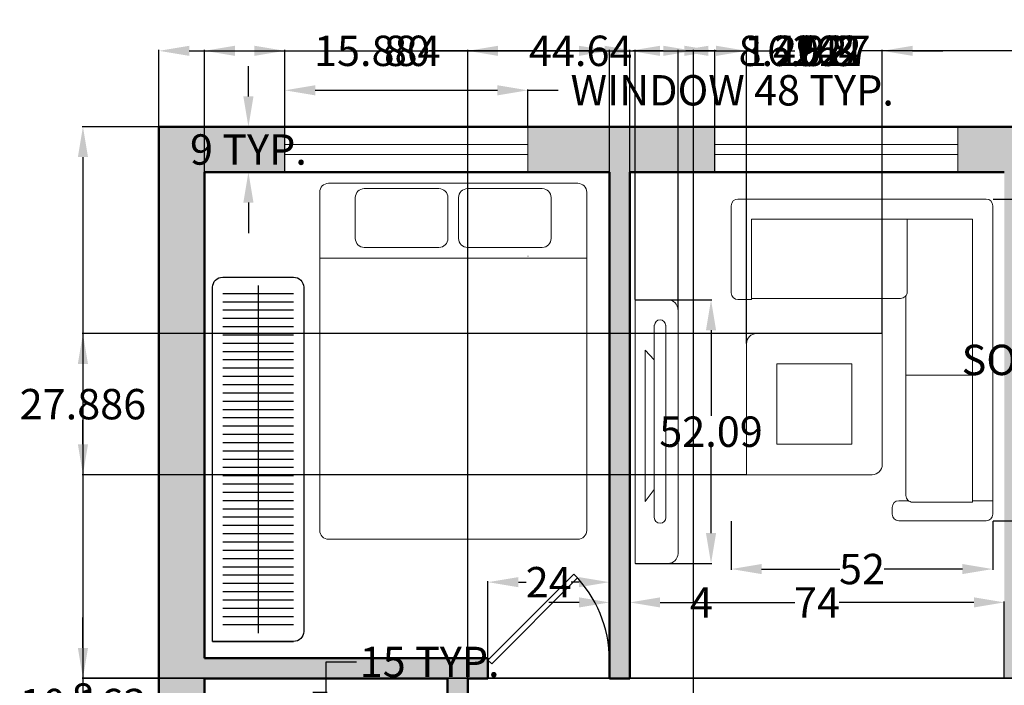
# Model space of a CAD drawing. Units: inches. Extents: x -11 to 341, y -300 to 41.
# Tile 3 of 5: x -3 to 192, y -91 to 41. Entities that reach past the tile are written whole.
import ezdxf

# ---------------------------------------------------------------- set-up
doc = ezdxf.new("R2010")
doc.units = ezdxf.units.IN
doc.header["$MEASUREMENT"] = 0
for name, color, linetype, lineweight in [('A-ANNO-DIMS', 2, 'Continuous', 18), ('A-DOOR', 3, 'Continuous', 25), ('A-FLOR-CASE', 8, 'Continuous', 25), ('A-FURN', 8, 'Continuous', 18), ('A-GLAZ', 4, 'Continuous', 18), ('A-WALL', 7, 'Continuous', 50), ('A-WALL-PATT', 251, 'Continuous', 13)]:
    doc.layers.add(name, color=color, linetype=linetype, lineweight=lineweight)
doc.styles.get("Standard").update_dxf_attribs({"font": 'arial.ttf'})
doc.dimstyles.get("Standard").update_dxf_attribs({"dimtxt": 6, "dimasz": 6, "dimexe": 0.18, "dimexo": 0.0625, "dimgap": 0.09, "dimtad": 0, "dimtih": 1, "dimtoh": 1, "dimdec": 0, "dimzin": 0, "dimdsep": 46, "dimlunit": 4, "dimtxsty": 'Standard', "dimcen": 0.09, "dimadec": 0, "dimazin": 0, "dimtfac": 1, "dimtdec": 0, "dimtofl": 0, "dimtmove": 0, "dimatfit": 3, "dimfxl": 1, "dimtolj": 1, "dimtzin": 0, "dimarcsym": 0})

# ---------------------------------------------------------------- blocks, each defined once
blk = doc.blocks.new('*U14')
for p, q in [((0, 0), (0, -6)), ((40, 0), (40, -6))]:
    blk.add_line(p, q)
blk.add_lwpolyline([(0, 0), (28.28, 28.28), (29.52, 27.05), (1.24, -1.24)], close=True)
blk.add_arc((0, 0), 40, 0, 45)
blk = doc.blocks.new('Bed - Queen')
for p, q in [((2, 0), (57.99999, 0)), ((0, -78.00003), (0, -2)), ((9.99999, -1.2), (26.79998, -1.2)), ((33.19999, -1.2), (49.99999, -1.2)), ((59.99999, -2), (59.99999, -78.00003)), ((7.99999, -12.4), (7.99999, -3.2)), ((28.79998, -3.2), (28.79998, -12.4)), ((31.19999, -12.4), (31.19999, -3.2)), ((51.99999, -3.2), (51.99999, -12.4)), ((9.99999, -14.4), (26.79998, -14.4)), ((33.19999, -14.4), (49.99999, -14.4)), ((59.99999, -16.8), (0, -16.8)), ((46.8, -16.4), (46.79936, -16.4)), ((57.99999, -80.00003), (2, -80.00003))]:
    blk.add_line(p, q)
for centre, start, end in [((2, -2), 90, 180), ((57.99999, -2), 0, 90), ((9.99999, -3.2), 90, 180), ((26.79998, -3.2), 0, 90), ((33.19999, -3.2), 90, 180), ((49.99999, -3.2), 0, 90), ((9.99999, -12.4), 180, 270), ((26.79998, -12.4), 270, 0), ((33.19999, -12.4), 180, 270), ((49.99999, -12.4), 270, 0), ((2, -78.00003), 180, 270), ((57.99999, -78.00003), 270, 0)]:
    blk.add_arc(centre, 2, start, end)
blk = doc.blocks.new('L Sofa')
for p, q in [((2, 30), (72, 30)), ((72, 30), (76, 30)), ((0, 24), (0, 28)), ((78, 28), (78, -54)), ((0, 2), (0, 24)), ((72, 24), (6, 24)), ((6, 24), (6, 0)), ((72, 24), (52.59, 24)), ((72, -60), (72, 24)), ((72, -22.55), (72, 24)), ((6, 0), (2, 0)), ((52.09, -22.55), (52.09, 1.16)), ((52.59, -22.55), (72, -22.55)), ((78, -54), (78, -60)), ((50, -60), (52.83, -60)), ((78, -60), (72, -60)), ((78, -60), (78, -64)), ((48, -64), (48, -62)), ((54, -66), (50, -66)), ((76, -66), (54, -66))]:
    blk.add_line(p, q)
for points in [[(6, 24), (52.48, 24), (52.48, 2.35, -0.414214), (50.48, 0.35), (6, 0.35)], [(72, -22.55), (52.09, -22.55), (52.09, -58.44, 0.414214), (54.09, -60.44), (72, -60.44)]]:
    blk.add_lwpolyline(points, format="xyb", close=True)
for centre, start, end in [((2, 28), 90, 180), ((76, 28), 0, 90), ((2, 2), 180, 270), ((50, -62), 90, 180), ((50, -64), 180, 270), ((76, -64), 270, 0)]:
    blk.add_arc(centre, 2, start, end)
blk = doc.blocks.new('WIN-48IN')
for p, q in [((0, 0), (0, 9)), ((48, 9), (48, 0)), ((0, 5.5), (48, 5.5)), ((0, 3.5), (48, 3.5))]:
    blk.add_line(p, q)
blk = doc.blocks.new('WARDROBE-HANGING-RAIL')
for p, q in [((7, 68.73), (7, 0)), ((14, 67.09), (0, 67.09)), ((14, 65.45), (0, 65.45)), ((14, 63.82), (0, 63.82)), ((14, 62.18), (0, 62.18)), ((14, 60.55), (0, 60.55)), ((14, 58.91), (0, 58.91)), ((14, 57.27), (0, 57.27)), ((14, 55.64), (0, 55.64)), ((14, 54), (0, 54)), ((14, 52.36), (0, 52.36)), ((14, 50.73), (0, 50.73)), ((14, 49.09), (0, 49.09)), ((14, 47.45), (0, 47.45)), ((14, 45.82), (0, 45.82)), ((14, 44.18), (0, 44.18)), ((14, 42.55), (0, 42.55)), ((14, 40.91), (0, 40.91)), ((14, 39.27), (0, 39.27)), ((14, 37.64), (0, 37.64)), ((14, 36), (0, 36)), ((14, 34.36), (0, 34.36)), ((14, 32.73), (0, 32.73)), ((14, 31.09), (0, 31.09)), ((14, 29.45), (0, 29.45)), ((14, 27.82), (0, 27.82)), ((14, 26.18), (0, 26.18)), ((14, 24.55), (0, 24.55)), ((14, 22.91), (0, 22.91)), ((14, 21.27), (0, 21.27)), ((14, 19.64), (0, 19.64)), ((14, 18), (0, 18)), ((14, 16.36), (0, 16.36)), ((14, 14.73), (0, 14.73)), ((14, 13.09), (0, 13.09)), ((14, 11.45), (0, 11.45)), ((14, 9.82), (0, 9.82)), ((14, 8.18), (0, 8.18)), ((14, 6.55), (0, 6.55)), ((14, 4.91), (0, 4.91)), ((14, 3.27), (0, 3.27)), ((14, 1.64), (0, 1.64))]:
    blk.add_line(p, q)
blk = doc.blocks.new('*D19')
at = {"layer": 'A-ANNO-DIMS', "color": 0, "lineweight": -2, "transparency": 16777216}
for p, q in [((49.45, 19.46), (49.45, 26.78)), ((55.45, 26.6), (91.45, 26.6)), ((97.45, 19.46), (97.45, 26.78)), ((97.45, 26.6), (103.45, 26.6))]:
    blk.add_line(p, q, dxfattribs=at)
at = {"layer": 'A-ANNO-DIMS', "color": 0, "transparency": 16777216}
for points in [[(55.45, 27.6), (55.45, 25.6), (49.45, 26.6)], [(91.45, 27.6), (91.45, 25.6), (97.45, 26.6)]]:
    blk.add_solid(points, dxfattribs=at)
at = {"layer": 'Defpoints', "color": 0, "transparency": 16777216}
for p in [(97.45, 26.6), (49.45, 19.4), (97.45, 19.4)]:
    blk.add_point(p, dxfattribs=at)
at = {"layer": 'A-ANNO-DIMS', "color": 0, "transparency": 16777216, "insert": (137.82, 26.6), "char_height": 6, "attachment_point": 5}
blk.add_mtext('\\A1;WINDOW 48 TYP.', dxfattribs=at)
blk = doc.blocks.new('*D20')
at = {"layer": 'A-ANNO-DIMS', "color": 0, "lineweight": -2, "transparency": 16777216}
for p, q in [((42.25, 25.4), (42.25, 31.4)), ((49.39, 19.4), (42.07, 19.4)), ((49.39, 10.4), (42.07, 10.4)), ((42.25, 4.4), (42.25, -1.6))]:
    blk.add_line(p, q, dxfattribs=at)
at = {"layer": 'A-ANNO-DIMS', "color": 0, "transparency": 16777216}
for points in [[(41.25, 25.4), (43.25, 25.4), (42.25, 19.4)], [(41.25, 4.4), (43.25, 4.4), (42.25, 10.4)]]:
    blk.add_solid(points, dxfattribs=at)
at = {"layer": 'Defpoints', "color": 0, "transparency": 16777216}
for p in [(42.25, 19.4), (49.45, 19.4), (49.45, 10.4)]:
    blk.add_point(p, dxfattribs=at)
at = {"layer": 'A-ANNO-DIMS', "color": 0, "transparency": 16777216, "insert": (42.25, 14.9), "char_height": 6, "attachment_point": 5}
blk.add_mtext('\\A1;9 TYP.', dxfattribs=at)
blk = doc.blocks.new('*D32')
at = {"layer": 'A-ANNO-DIMS', "color": 0, "lineweight": -2, "transparency": 16777216}
for p, q in [((57.63, -92.36), (57.63, -86.36)), ((57.63, -86.36), (63.63, -86.36)), ((54.99, -92.36), (57.81, -92.36)), ((57.63, -101.17), (57.63, -98.36)), ((54.99, -107.17), (57.81, -107.17))]:
    blk.add_line(p, q, dxfattribs=at)
at = {"layer": 'A-ANNO-DIMS', "color": 0, "transparency": 16777216}
for points in [[(56.63, -98.36), (58.63, -98.36), (57.63, -92.36)], [(56.63, -101.17), (58.63, -101.17), (57.63, -107.17)]]:
    blk.add_solid(points, dxfattribs=at)
at = {"layer": 'Defpoints', "color": 0, "transparency": 16777216}
for p in [(54.93, -92.36), (57.63, -92.36), (54.93, -107.17)]:
    blk.add_point(p, dxfattribs=at)
at = {"layer": 'A-ANNO-DIMS', "color": 0, "transparency": 16777216, "insert": (78.05, -86.36), "char_height": 6, "attachment_point": 5}
blk.add_mtext('\\A1;15 TYP.', dxfattribs=at)
blk = doc.blocks.new('*D41')
at = {"layer": 'A-ANNO-DIMS', "color": 0, "lineweight": -2, "transparency": 16777216}
for p, q in [((189.35, 5.11), (199, 5.11)), ((198.82, -0.89), (198.82, -23.48)), ((198.82, -52.47), (198.82, -29.87)), ((189.35, -58.47), (199, -58.47))]:
    blk.add_line(p, q, dxfattribs=at)
at = {"layer": 'A-ANNO-DIMS', "color": 0, "transparency": 16777216}
for points in [[(197.82, -0.89), (199.82, -0.89), (198.82, 5.11)], [(197.82, -52.47), (199.82, -52.47), (198.82, -58.47)]]:
    blk.add_solid(points, dxfattribs=at)
at = {"layer": 'Defpoints', "color": 0, "transparency": 16777216}
for p in [(189.29, 5.11), (198.82, 5.11), (189.29, -58.47)]:
    blk.add_point(p, dxfattribs=at)
at = {"layer": 'A-ANNO-DIMS', "color": 0, "transparency": 16777216, "insert": (198.82, -26.68), "char_height": 6, "attachment_point": 5}
blk.add_mtext('\\A1;SOFA 64', dxfattribs=at)
blk = doc.blocks.new('*D42')
at = {"layer": 'A-ANNO-DIMS', "color": 0, "lineweight": -2, "transparency": 16777216}
for p, q in [((137.63, -58.53), (137.63, -68.19)), ((189.29, -58.53), (189.29, -68.19)), ((143.63, -68.01), (159.1, -68.01)), ((183.29, -68.01), (167.81, -68.01))]:
    blk.add_line(p, q, dxfattribs=at)
at = {"layer": 'A-ANNO-DIMS', "color": 0, "transparency": 16777216}
for points in [[(143.63, -67.01), (143.63, -69.01), (137.63, -68.01)], [(183.29, -67.01), (183.29, -69.01), (189.29, -68.01)]]:
    blk.add_solid(points, dxfattribs=at)
at = {"layer": 'Defpoints', "color": 0, "transparency": 16777216}
for p in [(137.63, -58.47), (189.29, -58.47), (189.29, -68.01)]:
    blk.add_point(p, dxfattribs=at)
at = {"layer": 'A-ANNO-DIMS', "color": 0, "transparency": 16777216, "insert": (163.46, -68.01), "char_height": 6, "attachment_point": 5}
blk.add_mtext('\\A1;52', dxfattribs=at)
blk = doc.blocks.new('*D45')
at = {"layer": 'A-ANNO-DIMS', "color": 0, "lineweight": -2, "transparency": 16777216}
for p, q in [((24.57, 19.46), (24.57, 34.58)), ((30.57, 34.4), (149.81, 34.4)), ((282.57, 34.4), (163.32, 34.4)), ((288.57, 19.46), (288.57, 34.58))]:
    blk.add_line(p, q, dxfattribs=at)
at = {"layer": 'A-ANNO-DIMS', "color": 0, "transparency": 16777216}
for points in [[(30.57, 35.4), (30.57, 33.4), (24.57, 34.4)], [(282.57, 35.4), (282.57, 33.4), (288.57, 34.4)]]:
    blk.add_solid(points, dxfattribs=at)
at = {"layer": 'Defpoints', "color": 0, "transparency": 16777216}
for p in [(288.57, 34.4), (24.57, 19.4), (288.57, 19.4)]:
    blk.add_point(p, dxfattribs=at)
at = {"layer": 'A-ANNO-DIMS', "color": 0, "transparency": 16777216, "insert": (156.57, 34.4), "char_height": 6, "attachment_point": 5}
blk.add_mtext('\\A1;264', dxfattribs=at)
blk = doc.blocks.new('*D46')
at = {"layer": 'A-ANNO-DIMS', "color": 0, "lineweight": -2, "transparency": 16777216}
for p, q in [((24.5, 19.4), (9.38, 19.4)), ((9.56, 13.4), (9.56, -127.45)), ((9.56, -274.6), (9.56, -133.76)), ((24.5, -280.6), (9.38, -280.6))]:
    blk.add_line(p, q, dxfattribs=at)
at = {"layer": 'A-ANNO-DIMS', "color": 0, "transparency": 16777216}
for points in [[(8.56, 13.4), (10.56, 13.4), (9.56, 19.4)], [(8.56, -274.6), (10.56, -274.6), (9.56, -280.6)]]:
    blk.add_solid(points, dxfattribs=at)
at = {"layer": 'Defpoints', "color": 0, "transparency": 16777216}
for p in [(9.56, 19.4), (24.57, 19.4), (24.57, -280.6)]:
    blk.add_point(p, dxfattribs=at)
at = {"layer": 'A-ANNO-DIMS', "color": 0, "transparency": 16777216, "insert": (9.56, -130.6), "char_height": 6, "attachment_point": 5}
blk.add_mtext('\\A1;300', dxfattribs=at)
blk = doc.blocks.new('*D47')
at = {"layer": 'A-ANNO-DIMS', "color": 0, "lineweight": -2, "transparency": 16777216}
for p, q in [((33.57, 10.46), (33.57, 34.58)), ((39.57, 34.4), (43.45, 34.4)), ((49.45, 10.46), (49.45, 34.58)), ((49.45, 34.4), (55.45, 34.4))]:
    blk.add_line(p, q, dxfattribs=at)
at = {"layer": 'A-ANNO-DIMS', "color": 0, "transparency": 16777216}
for points in [[(39.57, 35.4), (39.57, 33.4), (33.57, 34.4)], [(43.45, 35.4), (43.45, 33.4), (49.45, 34.4)]]:
    blk.add_solid(points, dxfattribs=at)
at = {"layer": 'Defpoints', "color": 0, "transparency": 16777216}
for p in [(49.45, 34.4), (33.57, 10.4), (49.45, 10.4)]:
    blk.add_point(p, dxfattribs=at)
at = {"layer": 'A-ANNO-DIMS', "color": 0, "transparency": 16777216, "insert": (67.7, 34.4), "char_height": 6, "attachment_point": 5}
blk.add_mtext('\\A1;15.884', dxfattribs=at)
blk = doc.blocks.new('*D48')
at = {"layer": 'A-ANNO-DIMS', "color": 0, "lineweight": -2, "transparency": 16777216}
for p, q in [((117.57, 10.46), (117.57, 34.58)), ((123.57, 34.4), (128.39, 34.4)), ((134.39, 10.46), (134.39, 34.58)), ((134.39, 34.4), (140.39, 34.4))]:
    blk.add_line(p, q, dxfattribs=at)
at = {"layer": 'A-ANNO-DIMS', "color": 0, "transparency": 16777216}
for points in [[(123.57, 35.4), (123.57, 33.4), (117.57, 34.4)], [(128.39, 35.4), (128.39, 33.4), (134.39, 34.4)]]:
    blk.add_solid(points, dxfattribs=at)
at = {"layer": 'Defpoints', "color": 0, "transparency": 16777216}
for p in [(134.39, 34.4), (117.57, 10.4), (134.39, 10.4)]:
    blk.add_point(p, dxfattribs=at)
at = {"layer": 'A-ANNO-DIMS', "color": 0, "transparency": 16777216, "insert": (152.65, 34.4), "char_height": 6, "attachment_point": 5}
blk.add_mtext('\\A1;16.827', dxfattribs=at)
blk = doc.blocks.new('*D54')
at = {"layer": 'A-ANNO-DIMS', "color": 0, "lineweight": -2, "transparency": 16777216}
for p, q in [((33.57, -85.54), (33.57, 34.58)), ((39.57, 34.4), (69.18, 34.4)), ((107.57, 34.4), (77.95, 34.4)), ((113.57, -85.54), (113.57, 34.58))]:
    blk.add_line(p, q, dxfattribs=at)
at = {"layer": 'A-ANNO-DIMS', "color": 0, "transparency": 16777216}
for points in [[(39.57, 35.4), (39.57, 33.4), (33.57, 34.4)], [(107.57, 35.4), (107.57, 33.4), (113.57, 34.4)]]:
    blk.add_solid(points, dxfattribs=at)
at = {"layer": 'Defpoints', "color": 0, "transparency": 16777216}
for p in [(113.57, 34.4), (33.57, -85.6), (113.57, -85.6)]:
    blk.add_point(p, dxfattribs=at)
at = {"layer": 'A-ANNO-DIMS', "color": 0, "transparency": 16777216, "insert": (73.57, 34.4), "char_height": 6, "attachment_point": 5}
blk.add_mtext('\\A1;80', dxfattribs=at)
blk = doc.blocks.new('*D55')
at = {"layer": 'A-ANNO-DIMS', "color": 0, "lineweight": -2, "transparency": 16777216}
for p, q in [((107.57, -74.6), (101.57, -74.6)), ((113.57, -89.54), (113.57, -74.42)), ((117.57, -89.54), (117.57, -74.42)), ((123.57, -74.6), (129.57, -74.6))]:
    blk.add_line(p, q, dxfattribs=at)
at = {"layer": 'A-ANNO-DIMS', "color": 0, "transparency": 16777216}
for points in [[(107.57, -73.6), (107.57, -75.6), (113.57, -74.6)], [(123.57, -73.6), (123.57, -75.6), (117.57, -74.6)]]:
    blk.add_solid(points, dxfattribs=at)
at = {"layer": 'Defpoints', "color": 0, "transparency": 16777216}
for p in [(117.57, -74.6), (113.57, -89.6), (117.57, -89.6)]:
    blk.add_point(p, dxfattribs=at)
at = {"layer": 'A-ANNO-DIMS', "color": 0, "transparency": 16777216, "insert": (131.73, -74.6), "char_height": 6, "attachment_point": 5}
blk.add_mtext('\\A1;4', dxfattribs=at)
blk = doc.blocks.new('*D56')
at = {"layer": 'A-ANNO-DIMS', "color": 0, "lineweight": -2, "transparency": 16777216}
for p, q in [((117.57, -89.54), (117.57, -74.42)), ((123.57, -74.6), (150.21, -74.6)), ((185.57, -74.6), (158.92, -74.6)), ((191.57, -89.54), (191.57, -74.42))]:
    blk.add_line(p, q, dxfattribs=at)
at = {"layer": 'A-ANNO-DIMS', "color": 0, "transparency": 16777216}
for points in [[(123.57, -73.6), (123.57, -75.6), (117.57, -74.6)], [(185.57, -73.6), (185.57, -75.6), (191.57, -74.6)]]:
    blk.add_solid(points, dxfattribs=at)
at = {"layer": 'Defpoints', "color": 0, "transparency": 16777216}
for p in [(191.57, -74.6), (117.57, -89.6), (191.57, -89.6)]:
    blk.add_point(p, dxfattribs=at)
at = {"layer": 'A-ANNO-DIMS', "color": 0, "transparency": 16777216, "insert": (154.57, -74.6), "char_height": 6, "attachment_point": 5}
blk.add_mtext('\\A1;74', dxfattribs=at)
blk = doc.blocks.new('*D62')
at = {"layer": 'A-ANNO-DIMS', "color": 0, "lineweight": -2, "transparency": 16777216}
for p, q in [((85.57, -175.54), (85.57, 34.58)), ((91.57, 34.4), (150.16, 34.4)), ((221.57, 34.4), (162.97, 34.4)), ((227.57, -175.54), (227.57, 34.58))]:
    blk.add_line(p, q, dxfattribs=at)
at = {"layer": 'A-ANNO-DIMS', "color": 0, "transparency": 16777216}
for points in [[(91.57, 35.4), (91.57, 33.4), (85.57, 34.4)], [(221.57, 35.4), (221.57, 33.4), (227.57, 34.4)]]:
    blk.add_solid(points, dxfattribs=at)
at = {"layer": 'Defpoints', "color": 0, "transparency": 16777216}
for p in [(227.57, 34.4), (85.57, -175.6), (227.57, -175.6)]:
    blk.add_point(p, dxfattribs=at)
at = {"layer": 'A-ANNO-DIMS', "color": 0, "transparency": 16777216, "insert": (156.57, 34.4), "char_height": 6, "attachment_point": 5}
blk.add_mtext('\\A1;142', dxfattribs=at)
blk = doc.blocks.new('*D66')
at = {"layer": 'A-ANNO-DIMS', "color": 0, "lineweight": -2, "transparency": 16777216}
for p, q in [((9.563121, -83.603265), (9.563121, -77.603265)), ((231.502621, -89.603265), (9.383121, -89.603265)), ((231.502621, -97.603265), (9.383121, -97.603265)), ((9.563121, -103.603265), (9.563121, -109.603265))]:
    blk.add_line(p, q, dxfattribs=at)
at = {"layer": 'A-ANNO-DIMS', "color": 0, "transparency": 16777216}
for points in [[(8.563121, -83.603265), (10.563121, -83.603265), (9.563121, -89.603265)], [(8.563121, -103.603265), (10.563121, -103.603265), (9.563121, -97.603265)]]:
    blk.add_solid(points, dxfattribs=at)
at = {"layer": 'Defpoints', "color": 0, "transparency": 16777216}
for p in [(231.565121, -89.603265), (9.563121, -97.603265), (231.565121, -97.603265)]:
    blk.add_point(p, dxfattribs=at)
at = {"layer": 'A-ANNO-DIMS', "color": 0, "transparency": 16777216, "insert": (9.563121, -93.603265), "char_height": 6, "attachment_point": 5}
blk.add_mtext('\\A1;8', dxfattribs=at)
blk = doc.blocks.new('*D68')
at = {"layer": 'A-ANNO-DIMS', "color": 0, "lineweight": -2, "transparency": 16777216}
for p, q in [((89.57, -85.54), (89.57, -70.42)), ((95.57, -70.6), (97.14, -70.6)), ((107.57, -70.6), (105.99, -70.6)), ((113.57, -85.54), (113.57, -70.42))]:
    blk.add_line(p, q, dxfattribs=at)
at = {"layer": 'A-ANNO-DIMS', "color": 0, "transparency": 16777216}
for points in [[(95.57, -69.6), (95.57, -71.6), (89.57, -70.6)], [(107.57, -69.6), (107.57, -71.6), (113.57, -70.6)]]:
    blk.add_solid(points, dxfattribs=at)
at = {"layer": 'Defpoints', "color": 0, "transparency": 16777216}
for p in [(113.57, -70.6), (89.57, -85.6), (113.57, -85.6)]:
    blk.add_point(p, dxfattribs=at)
at = {"layer": 'A-ANNO-DIMS', "color": 0, "transparency": 16777216, "insert": (101.57, -70.6), "char_height": 6, "attachment_point": 5}
blk.add_mtext('\\A1;24', dxfattribs=at)
blk = doc.blocks.new('*D78')
at = {"layer": 'A-ANNO-DIMS', "color": 0, "lineweight": -2, "transparency": 16777216}
for p, q in [((118.69, -14.81), (133.81, -14.81)), ((133.63, -20.81), (133.63, -37.71)), ((133.63, -60.9), (133.63, -44.01)), ((118.69, -66.9), (133.81, -66.9))]:
    blk.add_line(p, q, dxfattribs=at)
at = {"layer": 'A-ANNO-DIMS', "color": 0, "transparency": 16777216}
for points in [[(132.63, -20.81), (134.63, -20.81), (133.63, -14.81)], [(132.63, -60.9), (134.63, -60.9), (133.63, -66.9)]]:
    blk.add_solid(points, dxfattribs=at)
at = {"layer": 'Defpoints', "color": 0, "transparency": 16777216}
for p in [(118.63, -14.81), (118.63, -66.9), (133.63, -66.9)]:
    blk.add_point(p, dxfattribs=at)
at = {"layer": 'A-ANNO-DIMS', "color": 0, "transparency": 16777216, "insert": (133.63, -40.86), "char_height": 6, "attachment_point": 5}
blk.add_mtext('\\A1;52.09', dxfattribs=at)
blk = doc.blocks.new('*D79')
at = {"layer": 'A-ANNO-DIMS', "color": 0, "lineweight": -2, "transparency": 16777216}
for p, q in [((112.63, 34.4), (106.63, 34.4)), ((118.63, -14.75), (118.63, 34.58)), ((127.12, -16.75), (127.12, 34.58)), ((133.12, 34.4), (139.12, 34.4))]:
    blk.add_line(p, q, dxfattribs=at)
at = {"layer": 'A-ANNO-DIMS', "color": 0, "transparency": 16777216}
for points in [[(112.63, 35.4), (112.63, 33.4), (118.63, 34.4)], [(133.12, 35.4), (133.12, 33.4), (127.12, 34.4)]]:
    blk.add_solid(points, dxfattribs=at)
at = {"layer": 'Defpoints', "color": 0, "transparency": 16777216}
for p in [(127.12, 34.4), (118.63, -14.81), (127.12, -16.81)]:
    blk.add_point(p, dxfattribs=at)
at = {"layer": 'A-ANNO-DIMS', "color": 0, "transparency": 16777216, "insert": (149.3, 34.4), "char_height": 6, "attachment_point": 5}
blk.add_mtext('\\A1;8.492', dxfattribs=at)
blk = doc.blocks.new('*D80')
at = {"layer": 'A-ANNO-DIMS', "color": 0, "lineweight": -2, "transparency": 16777216}
for p, q in [((134.645775, 34.398735), (128.645775, 34.398735)), ((140.645775, -23.409984), (140.645775, 34.578735)), ((167.445879, -21.409984), (167.445879, 34.578735)), ((173.445879, 34.398735), (179.445879, 34.398735))]:
    blk.add_line(p, q, dxfattribs=at)
at = {"layer": 'A-ANNO-DIMS', "color": 0, "transparency": 16777216}
for points in [[(134.645775, 35.398735), (134.645775, 33.398735), (140.645775, 34.398735)], [(173.445879, 35.398735), (173.445879, 33.398735), (167.445879, 34.398735)]]:
    blk.add_solid(points, dxfattribs=at)
at = {"layer": 'Defpoints', "color": 0, "transparency": 16777216}
for p in [(167.445879, 34.398735), (167.445879, -21.472484), (140.645775, -23.472484)]:
    blk.add_point(p, dxfattribs=at)
at = {"layer": 'A-ANNO-DIMS', "color": 0, "transparency": 16777216, "insert": (154.045827, 34.398735), "char_height": 6, "attachment_point": 5}
blk.add_mtext('\\A1;26.8', dxfattribs=at)
blk = doc.blocks.new('*D81')
at = {"layer": 'A-ANNO-DIMS', "color": 0, "lineweight": -2, "transparency": 16777216}
for p, q in [((167.38, -21.47), (9.38, -21.47)), ((9.56, -27.47), (9.56, -32.26)), ((9.56, -43.36), (9.56, -38.57)), ((140.58, -49.36), (9.38, -49.36))]:
    blk.add_line(p, q, dxfattribs=at)
at = {"layer": 'A-ANNO-DIMS', "color": 0, "transparency": 16777216}
for points in [[(8.56, -27.47), (10.56, -27.47), (9.56, -21.47)], [(8.56, -43.36), (10.56, -43.36), (9.56, -49.36)]]:
    blk.add_solid(points, dxfattribs=at)
at = {"layer": 'Defpoints', "color": 0, "transparency": 16777216}
for p in [(9.56, -21.47), (167.45, -21.47), (140.65, -49.36)]:
    blk.add_point(p, dxfattribs=at)
at = {"layer": 'A-ANNO-DIMS', "color": 0, "transparency": 16777216, "insert": (9.56, -35.42), "char_height": 6, "attachment_point": 5}
blk.add_mtext('\\A1;27.886', dxfattribs=at)
blk = doc.blocks.new('*D84')
at = {"layer": 'A-ANNO-DIMS', "color": 0, "lineweight": -2, "transparency": 16777216}
for p, q in [((9.56, -83.6), (9.56, -77.6)), ((279.5, -89.6), (9.38, -89.6)), ((267.79, -99.77), (9.38, -99.77)), ((9.56, -105.77), (9.56, -111.77))]:
    blk.add_line(p, q, dxfattribs=at)
at = {"layer": 'A-ANNO-DIMS', "color": 0, "transparency": 16777216}
for points in [[(8.56, -83.6), (10.56, -83.6), (9.56, -89.6)], [(8.56, -105.77), (10.56, -105.77), (9.56, -99.77)]]:
    blk.add_solid(points, dxfattribs=at)
at = {"layer": 'Defpoints', "color": 0, "transparency": 16777216}
for p in [(9.56, -89.6), (279.57, -89.6), (267.86, -99.77)]:
    blk.add_point(p, dxfattribs=at)
at = {"layer": 'A-ANNO-DIMS', "color": 0, "transparency": 16777216, "insert": (9.56, -94.68), "char_height": 6, "attachment_point": 5}
blk.add_mtext('\\A1;10.163', dxfattribs=at)
blk = doc.blocks.new('*D85')
at = {"layer": 'A-ANNO-DIMS', "color": 0, "lineweight": -2, "transparency": 16777216}
for p, q in [((85.57, -127.54), (85.57, 34.58)), ((91.57, 34.4), (97.56, 34.4)), ((124.2, 34.4), (118.21, 34.4)), ((130.2, -129.38), (130.2, 34.58))]:
    blk.add_line(p, q, dxfattribs=at)
at = {"layer": 'A-ANNO-DIMS', "color": 0, "transparency": 16777216}
for points in [[(91.57, 35.4), (91.57, 33.4), (85.57, 34.4)], [(124.2, 35.4), (124.2, 33.4), (130.2, 34.4)]]:
    blk.add_solid(points, dxfattribs=at)
at = {"layer": 'Defpoints', "color": 0, "transparency": 16777216}
for p in [(130.2, 34.4), (85.57, -127.6), (130.2, -129.44)]:
    blk.add_point(p, dxfattribs=at)
at = {"layer": 'A-ANNO-DIMS', "color": 0, "transparency": 16777216, "insert": (107.88, 34.4), "char_height": 6, "attachment_point": 5}
blk.add_mtext('\\A1;44.64', dxfattribs=at)

msp = doc.modelspace()

# ---------------------------------------------------------------- hatches: boundary and pattern name
at = {"layer": 'A-WALL-PATT'}
h = msp.add_hatch(color=256, dxfattribs=at)
h.dxf.hatch_style = 1
h.paths.add_polyline_path([(33.5651, 10.3967), (49.4488, 10.3967), (49.4488, 19.3967), (24.5651, 19.3967), (24.5651, -114.096), (33.5651, -114.096), (33.5651, -89.6033), (81.5651, -89.6033), (81.5651, -97.6033), (85.5651, -97.6033), (85.5651, -89.6033), (89.5651, -89.6033), (89.5651, -86.0033), (89.5651, -85.6033), (33.5651, -85.6033)])
h = msp.add_hatch(color=256, dxfattribs=at)
h.dxf.hatch_style = 1
h.paths.add_polyline_path([(134.3924, 19.3967), (97.4488, 19.3967), (97.4488, 10.3967), (113.5651, 10.3967), (113.5651, -85.6033), (113.5651, -89.6033), (117.5651, -89.6033), (117.5651, 10.3967), (134.3924, 10.3967)])
h = msp.add_hatch(color=256, dxfattribs=at)
h.dxf.hatch_style = 1
h.paths.add_polyline_path([(216.4841, 19.3967), (182.3924, 19.3967), (182.3924, 10.3967), (191.5651, 10.3967), (191.5651, -89.6033), (195.5651, -89.6033), (195.5651, -85.1033), (195.5651, 10.3967), (216.4841, 10.3967)])

# ---------------------------------------------------------------- linework, layer by layer
at = {"layer": 'A-FLOR-CASE'}
msp.add_lwpolyline([(35.1696, -82.3305), (35.1696, -12.3305, -0.41421356), (37.1696, -10.3305), (51.1696, -10.3305, -0.41421356), (53.1696, -12.3305), (53.1696, -80.3305, -0.41421356), (51.1696, -82.3305), (35.1696, -82.3305), (51.1696, -82.3305)], format="xyb", dxfattribs=at)
at = {"layer": 'A-FURN'}
for p, q in [((120.6279, -24.763), (122.4152, -26.6555)), ((120.6279, -54.673), (122.4152, -52.2554))]:
    msp.add_line(p, q, dxfattribs=at)
for points in [[(118.6264, -14.8127), (125.1179, -14.8127, -0.41421356), (127.1179, -16.8127), (127.1179, -64.9044, -0.41421356), (125.1179, -66.9044), (118.6264, -66.9044)], [(142.6458, -21.4725), (167.4459, -21.4725), (167.4459, -47.3583, -0.41421356), (165.4459, -49.3583), (140.6458, -49.3583), (140.6458, -23.4725, -0.41421356)]]:
    msp.add_lwpolyline(points, format="xyb", close=True, dxfattribs=at)
for points in [[(122.4152, -57.8163), (122.4152, -19.8366), (122.4801, -19.8366)], [(124.6548, -19.8366), (124.7197, -19.8366), (124.7197, -57.8163)], [(120.6279, -24.763), (120.6279, -54.673)], [(122.4152, -54.673), (122.4152, -24.763)]]:
    msp.add_lwpolyline(points, dxfattribs=at)
msp.add_lwpolyline([(146.6458, -27.4725), (161.4459, -27.4725), (161.4459, -43.3583), (146.6458, -43.3583)], close=True, dxfattribs=at)
for centre, radius, start, end in [((123.5675, -19.8366), 1.0873, 0, 180), ((123.5675, -57.8163), 1.1523, 180, 0)]:
    msp.add_arc(centre, radius, start, end, dxfattribs=at)
at = {"layer": 'A-WALL'}
for p, q in [((33.5651, 10.3967), (113.5651, 10.3967)), ((33.5651, -85.6033), (33.5651, 10.3967)), ((113.5651, -85.6033), (113.5651, 10.3967)), ((117.5651, -89.6033), (117.5651, 10.3967)), ((117.5651, 10.3967), (191.5651, 10.3967)), ((33.5651, -85.6033), (89.5651, -85.6033)), ((89.5651, -85.6033), (89.5651, -89.6033)), ((113.5651, -85.6033), (113.5651, -89.6033)), ((33.5651, -89.6033), (81.5651, -89.6033)), ((33.5651, -175.6033), (33.5651, -89.6033)), ((81.5651, -97.6033), (81.5651, -89.6033)), ((85.5651, -89.6033), (89.5651, -89.6033)), ((85.5651, -97.6033), (85.5651, -89.6033)), ((113.5651, -89.6033), (117.5651, -89.6033))]:
    msp.add_line(p, q, dxfattribs=at)
msp.add_lwpolyline([(129.5651, -280.6033), (24.5651, -280.6033), (24.5651, 19.3967), (288.5651, 19.3967), (288.5651, -280.6033), (165.5651, -280.6033)], dxfattribs=at)

# ---------------------------------------------------------------- block references
at = {"layer": 'A-DOOR', "xscale": 0.6, "yscale": 0.6, "zscale": 0.6}
msp.add_blockref('*U14', (89.5651, -86.0033), dxfattribs=at)
at = {"layer": 'A-FLOR-CASE'}
msp.add_blockref('WARDROBE-HANGING-RAIL', (37.17, -80.694), dxfattribs=at)
at = {"layer": 'A-FURN'}
for name, p, xscale, yscale, zscale in [('Bed - Queen', (56.3295, 8.2189), 0.8792308548308669, 0.8792308548308669, 0.8792308548308669), ('L Sofa', (137.6262, -14.7562), 0.6623116105517008, 0.6623116105517008, 0.6623116105517008)]:
    msp.add_blockref(name, p, dxfattribs=dict(at, xscale=xscale, yscale=yscale, zscale=zscale))
at = {"layer": 'A-GLAZ'}
for p in [(49.4488, 10.397), (134.3924, 10.397)]:
    msp.add_blockref('WIN-48IN', p, dxfattribs=at)

# ---------------------------------------------------------------- dimensions: what is measured, and where the dimension line sits
at = {"layer": 'A-ANNO-DIMS'}
dim = msp.add_linear_dim(base=(97.4488, 26.5967), p1=(49.4488, 19.3967), p2=(97.4488, 19.3967), text='WINDOW <> TYP.', dimstyle='Standard', override={"dimdec": 0, "dimlfac": 1, "dimrnd": 0, "dimzin": 0, "dimdsep": 46, "dimlunit": 2}, dxfattribs=at)
dim.commit()
dim.dimension.update_dxf_attribs({"geometry": '*D19', "text_midpoint": (137.8178, 26.5967)})
for base, p1, p2, override, picture, middle in [((288.5651, 34.3987), (24.5651, 19.3967), (288.5651, 19.3967), {"dimdec": 0, "dimlfac": 1, "dimrnd": 0, "dimzin": 0, "dimdsep": 46, "dimlunit": 2}, '*D45', (156.5651, 34.3987)), ((49.4488, 34.3987), (33.5651, 10.3967), (49.4488, 10.3967), {"dimdec": 3, "dimlfac": 1, "dimrnd": 0, "dimzin": 0, "dimdsep": 46, "dimlunit": 2}, '*D47', (67.6985, 34.3987)), ((113.5651, 34.3987), (33.5651, -85.6033), (113.5651, -85.6033), {"dimdec": 0, "dimlfac": 1, "dimrnd": 0, "dimzin": 0, "dimdsep": 46, "dimlunit": 2}, '*D54', (73.5651, 34.3987)), ((227.5651, 34.3987), (85.5651, -175.6033), (227.5651, -175.6033), {"dimdec": 0, "dimlfac": 1, "dimrnd": 0, "dimzin": 0, "dimdsep": 46, "dimlunit": 2}, '*D62', (156.5651, 34.3987)), ((130.204, 34.3987), (85.5651, -127.6033), (130.204, -129.4394), {"dimdec": 2, "dimlfac": 1, "dimrnd": 0, "dimzin": 0, "dimdsep": 46, "dimlunit": 2}, '*D85', (107.8846, 34.3987)), ((127.11793, 34.39874), (118.62639, -14.81271), (127.11793, -16.81271), {"dimdec": 3, "dimlfac": 1, "dimrnd": 0, "dimzin": 0, "dimdsep": 46, "dimlunit": 2}, '*D79', (149.30479, 34.39874)), ((134.3924, 34.3987), (117.5651, 10.3967), (134.3924, 10.3967), {"dimdec": 3, "dimlfac": 1, "dimrnd": 0, "dimzin": 0, "dimdsep": 46, "dimlunit": 2}, '*D48', (152.6543, 34.3987)), ((167.4459, 34.3987), (140.6458, -23.4725), (167.4459, -21.4725), {"dimdec": 1, "dimlfac": 1, "dimrnd": 0, "dimzin": 0, "dimdsep": 46, "dimlunit": 2}, '*D80', (154.0458, 34.3987)), ((189.2865, -68.0061), (137.6262, -58.4688), (189.2865, -58.4688), {"dimdec": 0, "dimlfac": 1, "dimrnd": 0, "dimzin": 0, "dimdsep": 46, "dimlunit": 2}, '*D42', (163.4563, -68.0061)), ((113.5651, -70.6013), (89.5651, -85.6033), (113.5651, -85.6033), {"dimdec": 0, "dimlfac": 1, "dimrnd": 0, "dimzin": 0, "dimdsep": 46, "dimlunit": 2}, '*D68', (101.5651, -70.6013)), ((117.5651, -74.6013), (113.5651, -89.6033), (117.5651, -89.6033), {"dimdec": 0, "dimlfac": 1, "dimrnd": 0, "dimzin": 0, "dimdsep": 46, "dimlunit": 2}, '*D55', (131.7302, -74.6013)), ((191.5651, -74.6013), (117.5651, -89.6033), (191.5651, -89.6033), {"dimdec": 0, "dimlfac": 1, "dimrnd": 0, "dimzin": 0, "dimdsep": 46, "dimlunit": 2}, '*D56', (154.5651, -74.6013))]:
    dim = msp.add_linear_dim(base=base, p1=p1, p2=p2, dimstyle='Standard', override=override, dxfattribs=at)
    dim.commit()
    dim.dimension.update_dxf_attribs({"geometry": picture, "text_midpoint": middle})
for base, p1, p2, text, picture, middle in [((42.2488, 19.3967), (49.4488, 10.3967), (49.4488, 19.3967), '<> TYP.', '*D20', (42.2488, 14.8967)), ((198.8238, 5.1131), (189.2865, -58.4688), (189.2865, 5.1131), 'SOFA <>', '*D41', (198.8238, -26.6778)), ((57.6345, -92.3627), (54.9264, -107.1706), (54.9264, -92.3627), '<> TYP.', '*D32', (78.0451, -86.3627))]:
    dim = msp.add_linear_dim(base=base, p1=p1, p2=p2, angle=90, text=text, dimstyle='Standard', override={"dimdec": 0, "dimlfac": 1, "dimrnd": 0, "dimzin": 0, "dimdsep": 46, "dimlunit": 2}, dxfattribs=at)
    dim.commit()
    dim.dimension.update_dxf_attribs({"geometry": picture, "text_midpoint": middle})
for base, p1, p2, angle, override, picture, middle in [((9.5631, 19.3967), (24.5651, -280.6033), (24.5651, 19.3967), 90, {"dimdec": 0, "dimlfac": 1, "dimrnd": 0, "dimzin": 0, "dimdsep": 46, "dimlunit": 2}, '*D46', (9.5631, -130.6033)), ((133.6284, -66.9044), (118.6264, -14.8127), (118.6264, -66.9044), 270, {"dimdec": 2, "dimlfac": 1, "dimrnd": 0, "dimzin": 0, "dimdsep": 46, "dimlunit": 2}, '*D78', (133.6284, -40.8586)), ((9.5631, -21.4725), (140.6458, -49.3583), (167.4459, -21.4725), 90, {"dimdec": 3, "dimlfac": 1, "dimrnd": 0, "dimzin": 0, "dimdsep": 46, "dimlunit": 2}, '*D81', (9.5631, -35.4154)), ((9.5631, -89.6033), (267.8569, -99.7667), (279.5651, -89.6033), 90, {"dimdec": 3, "dimlfac": 1, "dimrnd": 0, "dimzin": 0, "dimdsep": 46, "dimlunit": 2}, '*D84', (9.5631, -94.685)), ((9.5631, -97.6033), (231.5651, -89.6033), (231.5651, -97.6033), 90, {"dimdec": 0, "dimlfac": 1, "dimrnd": 0, "dimzin": 0, "dimdsep": 46, "dimlunit": 2}, '*D66', (9.5631, -93.6033))]:
    dim = msp.add_linear_dim(base=base, p1=p1, p2=p2, angle=angle, dimstyle='Standard', override=override, dxfattribs=at)
    dim.commit()
    dim.dimension.update_dxf_attribs({"geometry": picture, "text_midpoint": middle})

doc.saveas('drawing.dxf')
